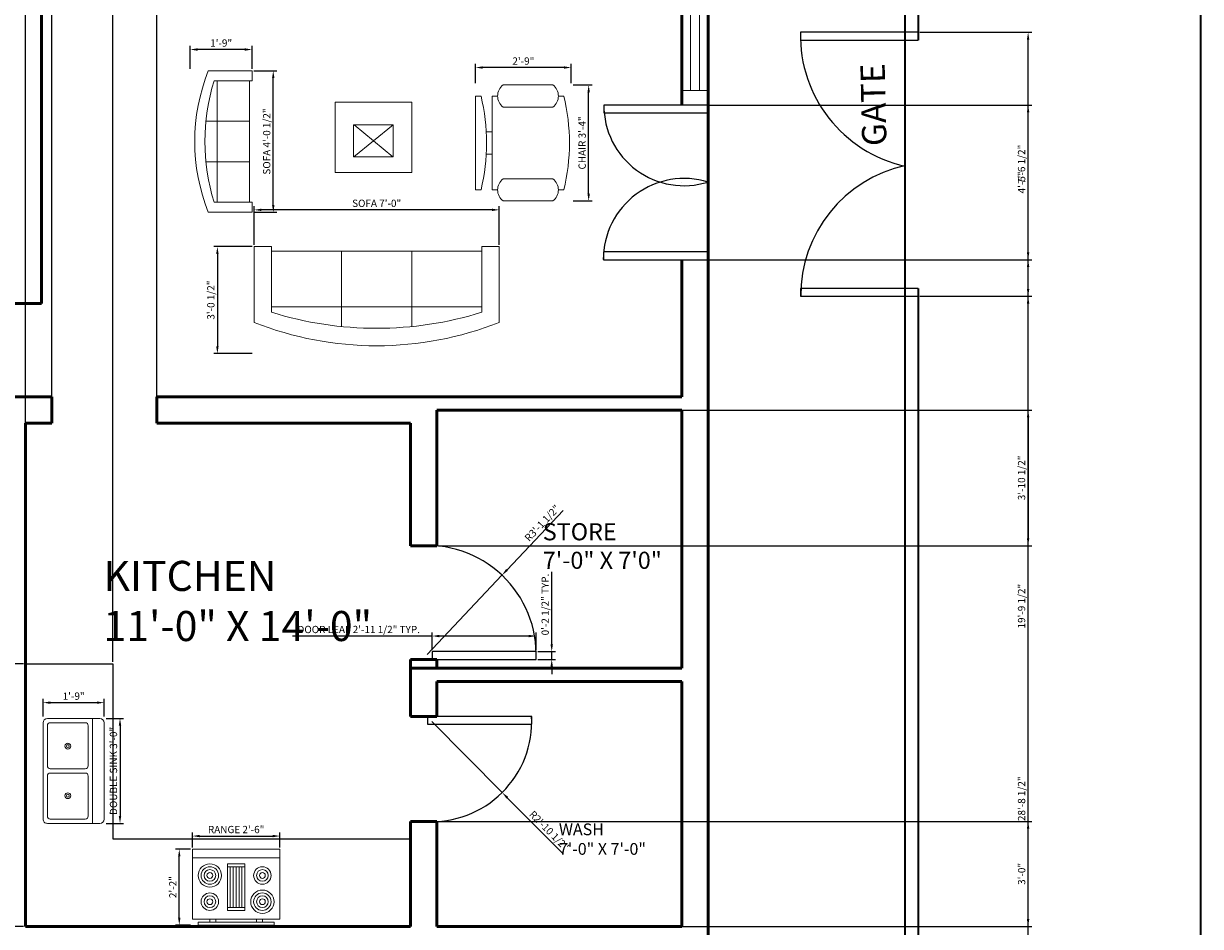
# Model space of a CAD drawing. Units: inches. Extents: x 65 to 818, y -87 to 880.
# Tile 4 of 6: x 414 to 818, y 148 to 457. Entities that reach past the tile are written whole.
import ezdxf

# ---------------------------------------------------------------- set-up
doc = ezdxf.new("R2010")
doc.units = ezdxf.units.IN
for name, color, linetype, lineweight in [('A-ANNO-DIMS', 2, 'Continuous', 18), ('A-ANNO-TEXT', 7, 'Continuous', 25), ('A-ANNO-TTLB', 7, 'Continuous', 35), ('A-AREA-IDEN', 7, 'Continuous', 25), ('A-DOOR', 3, 'Continuous', 25), ('A-EQPM', 9, 'Continuous', 18), ('A-FLOR-CASE', 32, 'Continuous', 25), ('A-FLOR-FIXT', 9, 'Continuous', 18), ('A-FURN', 8, 'Continuous', 18), ('A-GLAZ', 4, 'Continuous', 18), ('A-WALL', 7, 'Continuous', 50), ('C-PROP', 7, 'Continuous', 35), ('L-SITE-GATE', 3, 'Continuous', 25)]:
    doc.layers.add(name, color=color, linetype=linetype, lineweight=lineweight)
doc.styles.get("Standard").update_dxf_attribs({"font": 'arial.ttf'})
doc.dimstyles.new('ISO-25', dxfattribs={"dimtxt": 2.5, "dimasz": 2.5, "dimexe": 1.25, "dimexo": 0.625, "dimtad": 1, "dimtxsty": 'Standard', "dimcen": 2.5, "dimadec": 0, "dimazin": 0, "dimtfac": 1, "dimtmove": 0, "dimatfit": 3, "dimfxl": 1, "dimarcsym": 0})

# ---------------------------------------------------------------- blocks, each defined once
blk = doc.blocks.new('Range-Oven - 30 in top')
for p, q in [((0, -3), (30, -3)), ((12, -6), (18, -6)), ((13, -20), (13, -6)), ((14, -6), (14, -20)), ((15, -20), (15, -6)), ((16, -6), (16, -20)), ((17, -20), (17, -6)), ((18, -20), (12, -20)), ((6, -24), (6, -25)), ((8, -25), (8, -24)), ((22, -25), (22, -24)), ((24, -24), (24, -25))]:
    blk.add_line(p, q)
for points in [[(0, -24), (0, 0), (30, 0), (30, -24)], [(12, -21), (12, -5), (18, -5), (18, -21)], [(2, -26), (2, -25), (28, -25), (28, -26)]]:
    blk.add_lwpolyline(points, close=True)
for centre, radius in [((6, -9), 4), ((6, -9), 3), ((6, -9), 2), ((6, -9), 1), ((24, -9), 3), ((24, -9), 2), ((24, -9), 1), ((6, -18), 3), ((6, -18), 2), ((24, -18), 4), ((24, -18), 3), ((24, -18), 2), ((6, -18), 1), ((24, -18), 1)]:
    blk.add_circle(centre, radius)
blk = doc.blocks.new('Sink-double - 36 in top')
for p, q in [((-18, -4), (18, -4)), ((-0.75, -18.5), (-0.75, -6.5)), ((0.75, -6.5), (0.75, -18.5))]:
    blk.add_line(p, q)
for points in [[(-16.5, 0), (16.5, 0)], [(-18, -19.5), (-18, -1.5)], [(18, -1.5), (18, -19.5)], [(-16.5, -18.5), (-16.5, -6.5)], [(-15.5, -5.5), (-1.75, -5.5)], [(1.75, -5.5), (15.5, -5.5)], [(16.5, -6.5), (16.5, -18.5)], [(-1.75, -19.5), (-15.5, -19.5)], [(15.5, -19.5), (1.75, -19.5)], [(16.5, -21), (-16.5, -21)]]:
    blk.add_lwpolyline(points)
for centre, radius in [((-8.5, -12.5), 1), ((-8.5, -12.5), 0.5), ((8.5, -12.5), 1), ((8.5, -12.5), 0.5)]:
    blk.add_circle(centre, radius)
for centre, radius, start, end in [((-16.5, -1.5), 1.5, 90, 180), ((16.5, -1.5), 1.5, 0, 90), ((-15.5, -6.5), 1, 90, 180), ((-1.75, -6.5), 1, 0, 90), ((1.75, -6.5), 1, 90, 180), ((15.5, -6.5), 1, 0, 90), ((-16.5, -19.5), 1.5, 180, 270), ((-15.5, -18.5), 1, 180, 270), ((-1.75, -18.5), 1, 270, 0), ((1.75, -18.5), 1, 180, 270), ((15.5, -18.5), 1, 270, 0), ((16.5, -19.5), 1.5, 270, 0)]:
    blk.add_arc(centre, radius, start, end)
blk = doc.blocks.new('Sofa - Roundback 7 ft.')
for p, q in [((-12.00002, -32.4421), (-12.00003, -6.5971)), ((11.99997, -32.4421), (11.99998, -6.5971)), ((-36.000027, -34), (-36.000027, -11.4696)), ((35.99998, -34), (35.99998, -11.4696)), ((-35.999844, -13.3819), (35.9998, -13.3819)), ((-36.000027, -32.4421), (35.99998, -32.4421))]:
    blk.add_line(p, q)
for points in [[(-36.000027, -34), (-42.000027, -34), (-42.000027, -8)], [(41.99998, -8), (41.99998, -34), (35.99998, -34)]]:
    blk.add_lwpolyline(points)
for centre, radius, start, end in [((0, -114.25), 114.25, 68.43141, 111.5686), ((-0.00001, -127.1968), 121.1968, 72.72033, 107.2797)]:
    blk.add_arc(centre, radius, start, end)
blk = doc.blocks.new('Chair - Desk')
for p, q in [((-8.5, 0), (-8.5, -1)), ((-8.5, 0), (8.5, 0)), ((8.5, 0), (8.5, -1)), ((-2, -3), (-2, -1.9355)), ((2, -1.9576), (2, -3)), ((-8.5, -3), (-8.5, -4)), ((-8.5, -3), (8.5, -3)), ((8.5, -3), (8.5, -4)), ((-10.5, -5), (-10.5, -14)), ((-6.5, -14), (-6.5, -5)), ((6.5, -5), (6.5, -14)), ((10.5, -14), (10.5, -5)), ((-8.5, -15), (-8.5, -16)), ((8.5, -15), (8.5, -16))]:
    blk.add_line(p, q)
for centre, radius, start, end in [((0, 34.625), 36.625, 256.5803, 283.4197), ((-8.5, -6.5), 2.5, 36.8699, 143.1301), ((8.5, -6.5), 2.5, 36.8699, 143.1301), ((-8.5, -12.5), 2.5, 216.8699, 323.1301), ((8.5, -12.5), 2.5, 216.8699, 323.1301), ((0, 19.625), 36.625, 256.5803, 283.4197)]:
    blk.add_arc(centre, radius, start, end)
blk = doc.blocks.new('WIN-52X9-PLAN')
for p, q in [((9, 51.82), (0, 51.82)), ((0, 51.82), (0, 0)), ((3, 0), (3, 51.82)), ((6, 51.82), (6, 0)), ((9, 0), (9, 51.82)), ((0, 0), (9, 0))]:
    blk.add_line(p, q)
blk = doc.blocks.new('DOOR-LEAF-36-NOM')
blk.add_lwpolyline([(0, 0), (2.67, 0), (2.67, 35.67), (0, 35.67)], close=True)
blk = doc.blocks.new('*D18')
at = {"layer": 'A-ANNO-DIMS', "color": 0, "lineweight": -2, "transparency": 16777216}
for p, q in [((554.18, 247.07), (506.39, 247.07)), ((554.18, 242.34), (554.18, 248.32)), ((587.35, 247.07), (556.68, 247.07)), ((589.85, 242.34), (589.85, 248.32))]:
    blk.add_line(p, q, dxfattribs=at)
at = {"layer": 'A-ANNO-DIMS', "color": 0, "transparency": 16777216}
for points in [[(556.68, 247.48), (556.68, 246.65), (554.18, 247.07)], [(587.35, 247.48), (587.35, 246.65), (589.85, 247.07)]]:
    blk.add_solid(points, dxfattribs=at)
at = {"layer": 'Defpoints', "color": 0, "transparency": 16777216}
for p in [(554.18, 247.07), (554.18, 241.72), (589.85, 241.72)]:
    blk.add_point(p, dxfattribs=at)
at = {"layer": 'A-ANNO-DIMS', "color": 0, "transparency": 16777216, "insert": (529.04, 248.99), "char_height": 2.5, "attachment_point": 5}
blk.add_mtext('DOOR LEAF 2\'-11 1/2" TYP.', dxfattribs=at)
blk = doc.blocks.new('*D19')
at = {"layer": 'A-ANNO-DIMS', "color": 0, "lineweight": -2, "transparency": 16777216}
for p, q in [((595.2, 244.22), (595.2, 269.03)), ((590.47, 241.72), (596.45, 241.72)), ((590.47, 239.05), (596.45, 239.05)), ((595.2, 239.05), (595.2, 241.72)), ((595.2, 236.55), (595.2, 234.05))]:
    blk.add_line(p, q, dxfattribs=at)
at = {"layer": 'A-ANNO-DIMS', "color": 0, "transparency": 16777216}
for points in [[(594.78, 244.22), (595.61, 244.22), (595.2, 241.72)], [(594.78, 236.55), (595.61, 236.55), (595.2, 239.05)]]:
    blk.add_solid(points, dxfattribs=at)
at = {"layer": 'Defpoints', "color": 0, "transparency": 16777216}
for p in [(589.85, 241.72), (589.85, 239.05), (595.2, 241.72)]:
    blk.add_point(p, dxfattribs=at)
at = {"layer": 'A-ANNO-DIMS', "color": 0, "transparency": 16777216, "insert": (593.28, 257.87), "char_height": 2.5, "attachment_point": 5, "rotation": 90}
blk.add_mtext('0\'-2 1/2" TYP.', dxfattribs=at)
blk = doc.blocks.new('*D36')
at = {"layer": 'A-ANNO-DIMS', "color": 0, "lineweight": -2, "transparency": 16777216}
for p, q in [((493.19, 381.19), (493.19, 394.42)), ((574.69, 393.17), (495.69, 393.17)), ((577.19, 381.19), (577.19, 394.42))]:
    blk.add_line(p, q, dxfattribs=at)
at = {"layer": 'A-ANNO-DIMS', "color": 0, "transparency": 16777216}
for points in [[(495.69, 393.58), (495.69, 392.75), (493.19, 393.17)], [(574.69, 393.58), (574.69, 392.75), (577.19, 393.17)]]:
    blk.add_solid(points, dxfattribs=at)
at = {"layer": 'Defpoints', "color": 0, "transparency": 16777216}
for p in [(493.19, 393.17), (493.19, 380.57), (577.19, 380.57)]:
    blk.add_point(p, dxfattribs=at)
at = {"layer": 'A-ANNO-DIMS', "color": 0, "transparency": 16777216, "insert": (535.19, 395.08), "char_height": 2.5, "attachment_point": 5}
blk.add_mtext('SOFA 7\'-0"', dxfattribs=at)
blk = doc.blocks.new('*D37')
at = {"layer": 'A-ANNO-DIMS', "color": 0, "lineweight": -2, "transparency": 16777216}
for p, q in [((492.56, 380.57), (479.34, 380.57)), ((480.59, 378.07), (480.59, 346.4)), ((492.56, 343.9), (479.34, 343.9))]:
    blk.add_line(p, q, dxfattribs=at)
at = {"layer": 'A-ANNO-DIMS', "color": 0, "transparency": 16777216}
for points in [[(480.17, 378.07), (481.01, 378.07), (480.59, 380.57)], [(480.17, 346.4), (481.01, 346.4), (480.59, 343.9)]]:
    blk.add_solid(points, dxfattribs=at)
at = {"layer": 'Defpoints', "color": 0, "transparency": 16777216}
for p in [(493.19, 380.57), (480.59, 343.9), (493.19, 343.9)]:
    blk.add_point(p, dxfattribs=at)
at = {"layer": 'A-ANNO-DIMS', "color": 0, "transparency": 16777216, "insert": (478.67, 362.23), "char_height": 2.5, "attachment_point": 5, "rotation": 90}
blk.add_mtext('3\'-0 1/2"', dxfattribs=at)
blk = doc.blocks.new('*D38')
at = {"layer": 'A-ANNO-DIMS', "color": 0, "lineweight": -2, "transparency": 16777216}
for p, q in [((493.09, 440.84), (500.99, 440.84)), ((499.74, 394.83), (499.74, 438.34)), ((493.09, 392.33), (500.99, 392.33))]:
    blk.add_line(p, q, dxfattribs=at)
at = {"layer": 'A-ANNO-DIMS', "color": 0, "transparency": 16777216}
for points in [[(499.33, 438.34), (500.16, 438.34), (499.74, 440.84)], [(499.33, 394.83), (500.16, 394.83), (499.74, 392.33)]]:
    blk.add_solid(points, dxfattribs=at)
at = {"layer": 'Defpoints', "color": 0, "transparency": 16777216}
for p in [(492.47, 440.84), (499.74, 440.84), (492.47, 392.33)]:
    blk.add_point(p, dxfattribs=at)
at = {"layer": 'A-ANNO-DIMS', "color": 0, "transparency": 16777216, "insert": (497.82, 416.59), "char_height": 2.5, "attachment_point": 5, "rotation": 90}
blk.add_mtext('SOFA 4\'-0 1/2"', dxfattribs=at)
blk = doc.blocks.new('*D39')
at = {"layer": 'A-ANNO-DIMS', "color": 0, "lineweight": -2, "transparency": 16777216}
for p, q in [((471.29, 441.47), (471.29, 449.37)), ((489.97, 448.12), (473.79, 448.12)), ((492.47, 441.47), (492.47, 449.37))]:
    blk.add_line(p, q, dxfattribs=at)
at = {"layer": 'A-ANNO-DIMS', "color": 0, "transparency": 16777216}
for points in [[(473.79, 448.54), (473.79, 447.7), (471.29, 448.12)], [(489.97, 448.54), (489.97, 447.7), (492.47, 448.12)]]:
    blk.add_solid(points, dxfattribs=at)
at = {"layer": 'Defpoints', "color": 0, "transparency": 16777216}
for p in [(471.29, 448.12), (471.29, 440.84), (492.47, 440.84)]:
    blk.add_point(p, dxfattribs=at)
at = {"layer": 'A-ANNO-DIMS', "color": 0, "transparency": 16777216, "insert": (481.88, 450.02), "char_height": 2.5, "attachment_point": 5}
blk.add_mtext('1\'-9"', dxfattribs=at)
blk = doc.blocks.new('*D42')
at = {"layer": 'A-ANNO-DIMS', "color": 0, "lineweight": -2, "transparency": 16777216}
for p, q in [((472.02, 174.63), (472.02, 179.75)), ((474.52, 178.5), (499.52, 178.5)), ((502.02, 174.63), (502.02, 179.75))]:
    blk.add_line(p, q, dxfattribs=at)
at = {"layer": 'A-ANNO-DIMS', "color": 0, "transparency": 16777216}
for points in [[(474.52, 178.92), (474.52, 178.09), (472.02, 178.5)], [(499.52, 178.92), (499.52, 178.09), (502.02, 178.5)]]:
    blk.add_solid(points, dxfattribs=at)
at = {"layer": 'Defpoints', "color": 0, "transparency": 16777216}
for p in [(502.02, 178.5), (472.02, 174), (502.02, 174)]:
    blk.add_point(p, dxfattribs=at)
at = {"layer": 'A-ANNO-DIMS', "color": 0, "transparency": 16777216, "insert": (487.02, 180.42), "char_height": 2.5, "attachment_point": 5}
blk.add_mtext('RANGE 2\'-6"', dxfattribs=at)
blk = doc.blocks.new('*D43')
at = {"layer": 'A-ANNO-DIMS', "color": 0, "lineweight": -2, "transparency": 16777216}
for p, q in [((471.4, 174), (466.27, 174)), ((467.52, 150.5), (467.52, 171.5)), ((471.4, 148), (466.27, 148))]:
    blk.add_line(p, q, dxfattribs=at)
at = {"layer": 'A-ANNO-DIMS', "color": 0, "transparency": 16777216}
for points in [[(467.11, 171.5), (467.94, 171.5), (467.52, 174)], [(467.11, 150.5), (467.94, 150.5), (467.52, 148)]]:
    blk.add_solid(points, dxfattribs=at)
at = {"layer": 'Defpoints', "color": 0, "transparency": 16777216}
for p in [(467.52, 174), (472.02, 174), (472.02, 148)]:
    blk.add_point(p, dxfattribs=at)
at = {"layer": 'A-ANNO-DIMS', "color": 0, "transparency": 16777216, "insert": (465.64, 161), "char_height": 2.5, "attachment_point": 5, "rotation": 90}
blk.add_mtext('2\'-2"', dxfattribs=at)
blk = doc.blocks.new('*D44')
at = {"layer": 'A-ANNO-DIMS', "color": 0, "lineweight": -2, "transparency": 16777216}
for p, q in [((442.43, 218.84), (448.46, 218.84)), ((447.21, 216.34), (447.21, 185.34)), ((442.43, 182.84), (448.46, 182.84))]:
    blk.add_line(p, q, dxfattribs=at)
at = {"layer": 'A-ANNO-DIMS', "color": 0, "transparency": 16777216}
for points in [[(446.79, 216.34), (447.62, 216.34), (447.21, 218.84)], [(446.79, 185.34), (447.62, 185.34), (447.21, 182.84)]]:
    blk.add_solid(points, dxfattribs=at)
at = {"layer": 'Defpoints', "color": 0, "transparency": 16777216}
for p in [(441.81, 218.84), (441.81, 182.84), (447.21, 182.84)]:
    blk.add_point(p, dxfattribs=at)
at = {"layer": 'A-ANNO-DIMS', "color": 0, "transparency": 16777216, "insert": (445.29, 200.84), "char_height": 2.5, "attachment_point": 5, "rotation": 90}
blk.add_mtext('DOUBLE SINK 3\'-0"', dxfattribs=at)
blk = doc.blocks.new('*D45')
at = {"layer": 'A-ANNO-DIMS', "color": 0, "lineweight": -2, "transparency": 16777216}
for p, q in [((420.81, 219.46), (420.81, 225.49)), ((423.31, 224.24), (439.31, 224.24)), ((441.81, 219.46), (441.81, 225.49))]:
    blk.add_line(p, q, dxfattribs=at)
at = {"layer": 'A-ANNO-DIMS', "color": 0, "transparency": 16777216}
for points in [[(423.31, 224.65), (423.31, 223.82), (420.81, 224.24)], [(439.31, 224.65), (439.31, 223.82), (441.81, 224.24)]]:
    blk.add_solid(points, dxfattribs=at)
at = {"layer": 'Defpoints', "color": 0, "transparency": 16777216}
for p in [(441.81, 224.24), (420.81, 218.84), (441.81, 218.84)]:
    blk.add_point(p, dxfattribs=at)
at = {"layer": 'A-ANNO-DIMS', "color": 0, "transparency": 16777216, "insert": (431.31, 226.14), "char_height": 2.5, "attachment_point": 5}
blk.add_mtext('1\'-9"', dxfattribs=at)
blk = doc.blocks.new('*D46')
at = {"layer": 'A-ANNO-DIMS', "color": 0, "lineweight": -2, "transparency": 16777216}
for p, q in [((602.52, 435.98), (609.11, 435.98)), ((607.86, 398.7), (607.86, 433.48)), ((602.52, 396.2), (609.11, 396.2))]:
    blk.add_line(p, q, dxfattribs=at)
at = {"layer": 'A-ANNO-DIMS', "color": 0, "transparency": 16777216}
for points in [[(607.45, 433.48), (608.28, 433.48), (607.86, 435.98)], [(607.45, 398.7), (608.28, 398.7), (607.86, 396.2)]]:
    blk.add_solid(points, dxfattribs=at)
at = {"layer": 'Defpoints', "color": 0, "transparency": 16777216}
for p in [(601.9, 435.98), (607.86, 435.98), (601.9, 396.2)]:
    blk.add_point(p, dxfattribs=at)
at = {"layer": 'A-ANNO-DIMS', "color": 0, "transparency": 16777216, "insert": (605.95, 416.09), "char_height": 2.5, "attachment_point": 5, "rotation": 90}
blk.add_mtext('CHAIR 3\'-4"', dxfattribs=at)
blk = doc.blocks.new('*D47')
at = {"layer": 'A-ANNO-DIMS', "color": 0, "lineweight": -2, "transparency": 16777216}
for p, q in [((569.07, 436.6), (569.07, 443.2)), ((599.4, 441.95), (571.57, 441.95)), ((601.9, 436.6), (601.9, 443.2))]:
    blk.add_line(p, q, dxfattribs=at)
at = {"layer": 'A-ANNO-DIMS', "color": 0, "transparency": 16777216}
for points in [[(571.57, 442.36), (571.57, 441.53), (569.07, 441.95)], [(599.4, 442.36), (599.4, 441.53), (601.9, 441.95)]]:
    blk.add_solid(points, dxfattribs=at)
at = {"layer": 'Defpoints', "color": 0, "transparency": 16777216}
for p in [(569.07, 441.95), (569.07, 435.98), (601.9, 435.98)]:
    blk.add_point(p, dxfattribs=at)
at = {"layer": 'A-ANNO-DIMS', "color": 0, "transparency": 16777216, "insert": (585.48, 443.85), "char_height": 2.5, "attachment_point": 5}
blk.add_mtext('2\'-9"', dxfattribs=at)
blk = doc.blocks.new('*D55')
at = {"layer": 'A-ANNO-DIMS', "color": 0, "lineweight": -2, "transparency": 16777216}
for p, q in [((721.42, 454.02), (759.75, 454.02)), ((758.5, 366.05), (758.5, 451.52)), ((721.42, 363.55), (759.75, 363.55))]:
    blk.add_line(p, q, dxfattribs=at)
at = {"layer": 'A-ANNO-DIMS', "color": 0, "transparency": 16777216}
for points in [[(758.08, 451.52), (758.92, 451.52), (758.5, 454.02)], [(758.08, 366.05), (758.92, 366.05), (758.5, 363.55)]]:
    blk.add_solid(points, dxfattribs=at)
at = {"layer": 'Defpoints', "color": 0, "transparency": 16777216}
for p in [(720.8, 454.02), (758.5, 454.02), (720.8, 363.55)]:
    blk.add_point(p, dxfattribs=at)
at = {"layer": 'A-ANNO-DIMS', "color": 0, "transparency": 16777216, "insert": (756.58, 408.79), "char_height": 2.5, "attachment_point": 5, "rotation": 90}
blk.add_mtext('7\'-6 1/2"', dxfattribs=at)
blk = doc.blocks.new('*D56')
at = {"layer": 'A-ANNO-DIMS', "color": 0, "lineweight": -2, "transparency": 16777216}
for p, q in [((649.42, 429.07), (759.75, 429.07)), ((758.5, 378.58), (758.5, 426.57)), ((649.42, 376.08), (759.75, 376.08))]:
    blk.add_line(p, q, dxfattribs=at)
at = {"layer": 'A-ANNO-DIMS', "color": 0, "transparency": 16777216}
for points in [[(758.08, 426.57), (758.92, 426.57), (758.5, 429.07)], [(758.08, 378.58), (758.92, 378.58), (758.5, 376.08)]]:
    blk.add_solid(points, dxfattribs=at)
at = {"layer": 'Defpoints', "color": 0, "transparency": 16777216}
for p in [(648.8, 429.07), (758.5, 429.07), (648.8, 376.08)]:
    blk.add_point(p, dxfattribs=at)
at = {"layer": 'A-ANNO-DIMS', "color": 0, "transparency": 16777216, "insert": (756.6, 402.57), "char_height": 2.5, "attachment_point": 5, "rotation": 90}
blk.add_mtext('4\'-5"', dxfattribs=at)
blk = doc.blocks.new('*D58')
at = {"layer": 'A-ANNO-DIMS', "color": 0, "lineweight": -2, "transparency": 16777216}
for p, q in [((414.8, 238.17), (414.8, 777.99)), ((417.3, 776.74), (442.3, 776.74)), ((444.8, 238.17), (444.8, 777.99))]:
    blk.add_line(p, q, dxfattribs=at)
at = {"layer": 'A-ANNO-DIMS', "color": 0, "transparency": 16777216}
for points in [[(417.3, 777.16), (417.3, 776.32), (414.8, 776.74)], [(442.3, 777.16), (442.3, 776.32), (444.8, 776.74)]]:
    blk.add_solid(points, dxfattribs=at)
at = {"layer": 'Defpoints', "color": 0, "transparency": 16777216}
for p in [(444.8, 776.74), (414.8, 237.54), (444.8, 237.54)]:
    blk.add_point(p, dxfattribs=at)
at = {"layer": 'A-ANNO-DIMS', "color": 0, "transparency": 16777216, "insert": (429.8, 778.64), "char_height": 2.5, "attachment_point": 5}
blk.add_mtext('2\'-6"', dxfattribs=at)
blk = doc.blocks.new('*D60')
at = {"layer": 'A-ANNO-DIMS', "color": 0, "lineweight": -2, "transparency": 16777216}
for p, q in [((649.42, 376.08), (759.75, 376.08)), ((758.5, 141.04), (758.5, 373.58)), ((649.42, 138.54), (759.75, 138.54))]:
    blk.add_line(p, q, dxfattribs=at)
at = {"layer": 'A-ANNO-DIMS', "color": 0, "transparency": 16777216}
for points in [[(758.08, 373.58), (758.92, 373.58), (758.5, 376.08)], [(758.08, 141.04), (758.92, 141.04), (758.5, 138.54)]]:
    blk.add_solid(points, dxfattribs=at)
at = {"layer": 'Defpoints', "color": 0, "transparency": 16777216}
for p in [(648.8, 376.08), (758.5, 376.08), (648.8, 138.54)]:
    blk.add_point(p, dxfattribs=at)
at = {"layer": 'A-ANNO-DIMS', "color": 0, "transparency": 16777216, "insert": (756.58, 257.31), "char_height": 2.5, "attachment_point": 5, "rotation": 90}
blk.add_mtext('19\'-9 1/2"', dxfattribs=at)
blk = doc.blocks.new('*D65')
at = {"layer": 'A-ANNO-DIMS', "color": 0, "lineweight": -2, "transparency": 16777216}
for p, q in [((721.42, 363.55), (759.75, 363.55)), ((758.5, 21.54), (758.5, 361.05)), ((721.42, 19.04), (759.75, 19.04))]:
    blk.add_line(p, q, dxfattribs=at)
at = {"layer": 'A-ANNO-DIMS', "color": 0, "transparency": 16777216}
for points in [[(758.08, 361.05), (758.92, 361.05), (758.5, 363.55)], [(758.08, 21.54), (758.92, 21.54), (758.5, 19.04)]]:
    blk.add_solid(points, dxfattribs=at)
at = {"layer": 'Defpoints', "color": 0, "transparency": 16777216}
for p in [(720.8, 363.55), (758.5, 363.55), (720.8, 19.04)]:
    blk.add_point(p, dxfattribs=at)
at = {"layer": 'A-ANNO-DIMS', "color": 0, "transparency": 16777216, "insert": (756.58, 191.3), "char_height": 2.5, "attachment_point": 5, "rotation": 90}
blk.add_mtext('28\'-8 1/2"', dxfattribs=at)
blk = doc.blocks.new('*D66')
at = {"layer": 'A-ANNO-DIMS', "color": 0, "lineweight": -2, "transparency": 16777216}
for p, q in [((423.8, 320.67), (423.8, 777.99)), ((426.3, 776.74), (457.3, 776.74)), ((459.8, 320.67), (459.8, 777.99))]:
    blk.add_line(p, q, dxfattribs=at)
at = {"layer": 'A-ANNO-DIMS', "color": 0, "transparency": 16777216}
for points in [[(426.3, 777.16), (426.3, 776.32), (423.8, 776.74)], [(457.3, 777.16), (457.3, 776.32), (459.8, 776.74)]]:
    blk.add_solid(points, dxfattribs=at)
at = {"layer": 'Defpoints', "color": 0, "transparency": 16777216}
for p in [(459.8, 776.74), (423.8, 320.04), (459.8, 320.04)]:
    blk.add_point(p, dxfattribs=at)
at = {"layer": 'A-ANNO-DIMS', "color": 0, "transparency": 16777216, "insert": (441.8, 778.64), "char_height": 2.5, "attachment_point": 5}
blk.add_mtext('3\'-0"', dxfattribs=at)
blk = doc.blocks.new('*D69')
at = {"layer": 'A-ANNO-DIMS', "color": 0, "lineweight": -2, "transparency": 16777216}
for p, q in [((556.42, 183.54), (759.75, 183.54)), ((758.5, 150.04), (758.5, 181.04)), ((556.42, 147.54), (759.75, 147.54))]:
    blk.add_line(p, q, dxfattribs=at)
at = {"layer": 'A-ANNO-DIMS', "color": 0, "transparency": 16777216}
for points in [[(758.08, 181.04), (758.92, 181.04), (758.5, 183.54)], [(758.08, 150.04), (758.92, 150.04), (758.5, 147.54)]]:
    blk.add_solid(points, dxfattribs=at)
at = {"layer": 'Defpoints', "color": 0, "transparency": 16777216}
for p in [(555.8, 183.54), (758.5, 183.54), (555.8, 147.54)]:
    blk.add_point(p, dxfattribs=at)
at = {"layer": 'A-ANNO-DIMS', "color": 0, "transparency": 16777216, "insert": (756.6, 165.54), "char_height": 2.5, "attachment_point": 5, "rotation": 90}
blk.add_mtext('3\'-0"', dxfattribs=at)
blk = doc.blocks.new('*D70')
at = {"layer": 'A-ANNO-DIMS', "color": 0, "lineweight": -2, "transparency": 16777216}
for p, q in [((556.42, 324.54), (759.75, 324.54)), ((758.5, 322.04), (758.5, 280.54)), ((556.42, 278.04), (759.75, 278.04))]:
    blk.add_line(p, q, dxfattribs=at)
at = {"layer": 'A-ANNO-DIMS', "color": 0, "transparency": 16777216}
for points in [[(758.08, 322.04), (758.92, 322.04), (758.5, 324.54)], [(758.08, 280.54), (758.92, 280.54), (758.5, 278.04)]]:
    blk.add_solid(points, dxfattribs=at)
at = {"layer": 'Defpoints', "color": 0, "transparency": 16777216}
for p in [(555.8, 324.54), (555.8, 278.04), (758.5, 278.04)]:
    blk.add_point(p, dxfattribs=at)
at = {"layer": 'A-ANNO-DIMS', "color": 0, "transparency": 16777216, "insert": (756.58, 301.29), "char_height": 2.5, "attachment_point": 5, "rotation": 90}
blk.add_mtext('3\'-10 1/2"', dxfattribs=at)
blk = doc.blocks.new('*D74')
at = {"layer": 'A-ANNO-DIMS', "color": 0, "lineweight": -2, "transparency": 16777216}
for p, q in [((414.17, 237.54), (201.85, 237.54)), ((203.1, 150.04), (203.1, 235.04)), ((414.17, 147.54), (201.85, 147.54))]:
    blk.add_line(p, q, dxfattribs=at)
at = {"layer": 'A-ANNO-DIMS', "color": 0, "transparency": 16777216}
for points in [[(202.68, 235.04), (203.52, 235.04), (203.1, 237.54)], [(202.68, 150.04), (203.52, 150.04), (203.1, 147.54)]]:
    blk.add_solid(points, dxfattribs=at)
at = {"layer": 'Defpoints', "color": 0, "transparency": 16777216}
for p in [(203.1, 237.54), (414.8, 237.54), (414.8, 147.54)]:
    blk.add_point(p, dxfattribs=at)
at = {"layer": 'A-ANNO-DIMS', "color": 0, "transparency": 16777216, "insert": (201.2, 192.54), "char_height": 2.5, "attachment_point": 5, "rotation": 90}
blk.add_mtext('7\'-6"', dxfattribs=at)
blk = doc.blocks.new('*D78')
at = {"layer": 'A-ANNO-DIMS', "color": 0, "lineweight": -2, "transparency": 16777216}
for p, q in [((554.06, 217.78), (578.22, 193.43)), ((599.07, 172.4), (579.98, 191.65))]:
    blk.add_line(p, q, dxfattribs=at)
at = {"layer": 'A-ANNO-DIMS', "color": 0, "transparency": 16777216}
blk.add_solid([(580.27, 191.94), (579.68, 191.36), (578.22, 193.43)], dxfattribs=at)
at = {"layer": 'Defpoints', "color": 0, "transparency": 16777216}
for p in [(554.06, 217.78), (578.22, 193.43)]:
    blk.add_point(p, dxfattribs=at)
at = {"layer": 'A-ANNO-DIMS', "color": 0, "transparency": 16777216, "insert": (594.07, 180.16), "char_height": 2.5, "attachment_point": 5, "rotation": 314.7642}
blk.add_mtext('R2\'-10 1/2"', dxfattribs=at)
blk = doc.blocks.new('*D82')
at = {"layer": 'A-ANNO-DIMS', "color": 0, "lineweight": -2, "transparency": 16777216}
for p, q in [((599.09, 290.1), (579.87, 269.74)), ((552.47, 240.73), (578.15, 267.92))]:
    blk.add_line(p, q, dxfattribs=at)
at = {"layer": 'A-ANNO-DIMS', "color": 0, "transparency": 16777216}
blk.add_solid([(579.56, 270.03), (580.17, 269.45), (578.15, 267.92)], dxfattribs=at)
at = {"layer": 'Defpoints', "color": 0, "transparency": 16777216}
for p in [(578.15, 267.92), (552.47, 240.73)]:
    blk.add_point(p, dxfattribs=at)
at = {"layer": 'A-ANNO-DIMS', "color": 0, "transparency": 16777216, "insert": (592.16, 285.56), "char_height": 2.5, "attachment_point": 5, "rotation": 46.6417}
blk.add_mtext('R3\'-1 1/2"', dxfattribs=at)

msp = doc.modelspace()

# ---------------------------------------------------------------- linework, layer by layer
at = {"layer": 'A-ANNO-TTLB'}
msp.add_lwpolyline([(64.55, 880.46), (817.59, 880.46), (817.59, -87.37), (64.55, -87.37)], close=True, dxfattribs=at)
at = {"layer": 'A-DOOR'}
for points in [[(648.8, 429.07), (613.08, 429.07), (613.08, 426.4), (648.8, 426.41)], [(648.8, 378.74), (612.9, 378.74), (612.9, 376.08), (648.8, 376.08)]]:
    msp.add_lwpolyline(points, dxfattribs=at)
for centre, radius, start, end in [((640.55, 428.93), 27.49, 179.6774, 287.4638), ((640.61, 376.17), 27.75, 72.8481, 180.1098), ((552.47, 240.73), 37.41, 357.4133, 95.8708), ((554.06, 217.78), 34.3, 266.6167, 2.9116)]:
    msp.add_arc(centre, radius, start, end, dxfattribs=at)
at = {"layer": 'A-FLOR-CASE'}
for p, q in [((414.8, 237.54), (444.8, 237.54)), ((444.8, 237.54), (444.8, 177.54)), ((444.8, 177.54), (546.8, 177.54))]:
    msp.add_line(p, q, dxfattribs=at)
at = {"layer": 'A-FURN'}
for p, q in [((527.33, 411.31), (540.79, 422.27)), ((540.72, 411.35), (527.49, 422.28))]:
    msp.add_line(p, q, dxfattribs=at)
for points in [[(520.92, 430.08), (547.26, 430.08), (547.26, 405.92), (520.92, 405.92)], [(527.3, 422.28), (540.79, 422.28), (540.79, 411.35), (527.3, 411.35)]]:
    msp.add_lwpolyline(points, close=True, dxfattribs=at)
at = {"layer": 'A-WALL'}
for p, q in [((648.8, 703.04), (648.8, 138.54)), ((639.8, 517.04), (639.8, 429.07)), ((420.3, 361.04), (420.3, 460.04)), ((639.8, 402.69), (639.8, 402.69)), ((639.8, 376.08), (639.8, 329.04)), ((374.3, 361.04), (420.3, 361.04)), ((405.8, 329.04), (423.8, 329.04)), ((423.8, 329.04), (423.8, 320.04)), ((459.8, 329.04), (459.8, 320.04)), ((459.8, 329.04), (639.8, 329.04)), ((555.8, 324.54), (639.8, 324.54)), ((555.8, 324.54), (555.8, 278.04)), ((639.8, 324.54), (639.8, 236.04)), ((414.8, 320.04), (423.8, 320.04)), ((414.8, 320.04), (414.8, 147.54)), ((459.8, 320.04), (546.8, 320.04)), ((546.8, 320.04), (546.8, 278.04)), ((546.8, 278.04), (555.8, 278.04)), ((546.8, 239.04), (555.8, 239.04)), ((546.8, 239.04), (546.8, 219.54)), ((555.8, 239.04), (555.8, 236.04)), ((546.8, 236.04), (639.8, 236.04)), ((555.8, 231.54), (639.8, 231.54)), ((555.8, 231.54), (555.8, 219.54)), ((639.8, 231.54), (639.8, 147.54)), ((546.8, 219.54), (555.8, 219.54)), ((546.8, 183.54), (555.8, 183.54)), ((546.8, 183.54), (546.8, 147.54)), ((555.8, 183.54), (555.8, 147.54)), ((414.8, 147.54), (546.8, 147.54)), ((555.8, 147.54), (639.8, 147.54))]:
    msp.add_line(p, q, dxfattribs=at)
at = {"layer": 'C-PROP'}
for p, q in [((720.8, 739.04), (720.8, 451.35)), ((716.3, 734.54), (716.3, 23.54)), ((720.8, 366.22), (720.8, 19.04))]:
    msp.add_line(p, q, dxfattribs=at)
at = {"layer": 'L-SITE-GATE'}
for points in [[(720.8, 454.02), (680.47, 454.02), (680.47, 451.35), (720.8, 451.35)], [(720.8, 366.22), (680.47, 366.22), (680.47, 363.55), (720.8, 363.55)]]:
    msp.add_lwpolyline(points, dxfattribs=at)
for centre, radius, start, end in [((726.32, 452.93), 45.87, 178.7141, 257.4649), ((726.08, 363.86), 45.53, 102.1735, 180.4965)]:
    msp.add_arc(centre, radius, start, end, dxfattribs=at)

# ---------------------------------------------------------------- block references
at = {"layer": 'A-DOOR', "rotation": 90.00000000000007}
for p in [(589.85, 239.05), (588.34, 216.87)]:
    msp.add_blockref('DOOR-LEAF-36-NOM', p, dxfattribs=at)
at = {"layer": 'A-EQPM'}
msp.add_blockref('Range-Oven - 30 in top', (472.02, 174), dxfattribs=at)
at = {"layer": 'A-FLOR-FIXT', "rotation": 270}
msp.add_blockref('Sink-double - 36 in top', (441.81, 200.84), dxfattribs=at)
at = {"layer": 'A-FURN'}
for name, p, xscale, yscale, zscale, rotation in [('Sofa - Roundback 7 ft.', (472.83, 416.59), 0.5775366576221616, 0.5775366576221616, 0.5775366576221616, 89.99999999999999), ('Chair - Desk', (569.07, 416.09), 1.894169593508299, 1.894169593508299, 1.894169593508299, 90)]:
    msp.add_blockref(name, p, dxfattribs=dict(at, xscale=xscale, yscale=yscale, zscale=zscale, rotation=rotation))
at = {"layer": 'A-FURN', "rotation": 180}
msp.add_blockref('Sofa - Roundback 7 ft.', (535.19, 346.57), dxfattribs=at)
at = {"layer": 'A-GLAZ'}
msp.add_blockref('WIN-52X9-PLAN', (639.8, 434.13), dxfattribs=at)

# ---------------------------------------------------------------- texts
at = {"layer": 'A-ANNO-TEXT', "insert": (701.64, 414.94), "char_height": 8.353, "attachment_point": 1, "rotation": 91.3254}
msp.add_mtext_dynamic_manual_height_columns('GATE', width=13.7685, gutter_width=41.77, heights=[0], dxfattribs=at)
at = {"layer": 'A-AREA-IDEN', "attachment_point": 1}
for s, width, gutter_width, insert, char_height in [('STORE\\P7\'-0" X 7\'0"', 90.223, 29.37, (592.14, 285.76), 5.8749), ('KITCHEN\\P11\'-0" X 14\'-0"', 100.5512, 51.51, (441.56, 272.83), 10.3025), ('WASH\\P7\'-0" X 7\'-0"', 31.7279, 20.11, (597.66, 182.81), 4.0221)]:
    msp.add_mtext_dynamic_manual_height_columns(s, width=width, gutter_width=gutter_width, heights=[0], dxfattribs=dict(at, insert=insert, char_height=char_height))

# ---------------------------------------------------------------- dimensions: what is measured, and where the dimension line sits
at = {"layer": 'A-ANNO-DIMS'}
for base, p1, p2, picture, middle in [((444.8, 776.74), (414.8, 237.54), (444.8, 237.54), '*D58', (429.8, 778.64)), ((459.8, 776.74), (423.8, 320.04), (459.8, 320.04), '*D66', (441.8, 778.64)), ((441.81, 224.24), (420.81, 218.84), (441.81, 218.84), '*D45', (431.31, 226.14))]:
    dim = msp.add_linear_dim(base=base, p1=p1, p2=p2, dimstyle='ISO-25', override={"dimdec": 1, "dimlfac": 1, "dimrnd": 0, "dimzin": 1, "dimdsep": 46, "dimlunit": 4, "dimfrac": 2}, dxfattribs=at)
    dim.commit()
    dim.dimension.update_dxf_attribs({"geometry": picture, "text_midpoint": middle})
for base, p1, p2, angle, picture, middle in [((758.5, 454.02), (720.8, 363.55), (720.8, 454.02), 90, '*D55', (756.58, 408.79)), ((471.29, 448.12), (492.47, 440.84), (471.29, 440.84), 180, '*D39', (481.88, 450.02)), ((569.07, 441.95), (601.9, 435.98), (569.07, 435.98), 180, '*D47', (585.48, 443.85)), ((758.5, 429.07), (648.8, 376.08), (648.8, 429.07), 90, '*D56', (756.6, 402.57)), ((480.59, 343.9), (493.19, 380.57), (493.19, 343.9), 270, '*D37', (478.67, 362.23)), ((758.5, 376.08), (648.8, 138.54), (648.8, 376.08), 90, '*D60', (756.58, 257.31)), ((758.5, 363.55), (720.8, 19.04), (720.8, 363.55), 90, '*D65', (756.58, 191.3)), ((758.5, 278.04), (555.8, 324.54), (555.8, 278.04), 90, '*D70', (756.58, 301.29)), ((203.1, 237.54), (414.8, 147.54), (414.8, 237.54), 90, '*D74', (201.2, 192.54)), ((758.5, 183.54), (555.8, 147.54), (555.8, 183.54), 90, '*D69', (756.6, 165.54)), ((467.52, 174), (472.02, 148), (472.02, 174), 90, '*D43', (465.64, 161))]:
    dim = msp.add_linear_dim(base=base, p1=p1, p2=p2, angle=angle, dimstyle='ISO-25', override={"dimdec": 1, "dimlfac": 1, "dimrnd": 0, "dimzin": 1, "dimdsep": 46, "dimlunit": 4, "dimfrac": 2}, dxfattribs=at)
    dim.commit()
    dim.dimension.update_dxf_attribs({"geometry": picture, "text_midpoint": middle})
for base, p1, p2, angle, text, picture, middle in [((499.74, 440.84), (492.47, 392.33), (492.47, 440.84), 90, 'SOFA <>', '*D38', (497.82, 416.59)), ((607.86, 435.98), (601.9, 396.2), (601.9, 435.98), 90, 'CHAIR <>', '*D46', (605.95, 416.09)), ((493.19, 393.17), (577.19, 380.57), (493.19, 380.57), 180, 'SOFA <>', '*D36', (535.19, 395.08)), ((595.2, 241.72), (589.85, 239.05), (589.85, 241.72), 90, '<> TYP.', '*D19', (593.28, 257.87)), ((554.18, 247.07), (589.85, 241.72), (554.18, 241.72), 180, 'DOOR LEAF <> TYP.', '*D18', (529.04, 248.99)), ((447.21, 182.84), (441.81, 218.84), (441.81, 182.84), 270, 'DOUBLE SINK <>', '*D44', (445.29, 200.84))]:
    dim = msp.add_linear_dim(base=base, p1=p1, p2=p2, angle=angle, text=text, dimstyle='ISO-25', override={"dimdec": 1, "dimlfac": 1, "dimrnd": 0, "dimzin": 1, "dimdsep": 46, "dimlunit": 4, "dimfrac": 2}, dxfattribs=at)
    dim.commit()
    dim.dimension.update_dxf_attribs({"geometry": picture, "text_midpoint": middle})
for center, mpoint, picture, middle in [((552.47, 240.73), (578.15, 267.92), '*D82', (593.56, 284.24)), ((554.06, 217.78), (578.22, 193.43), '*D78', (592.71, 178.81))]:
    dim = msp.add_radius_dim(center=center, mpoint=mpoint, dimstyle='ISO-25', override={"dimdec": 1, "dimlfac": 1, "dimrnd": 0, "dimzin": 1, "dimdsep": 46, "dimlunit": 4, "dimfrac": 2}, dxfattribs=at)
    dim.commit()
    dim.dimension.update_dxf_attribs({"geometry": picture, "text_midpoint": middle, "dimtype": 164})
dim = msp.add_linear_dim(base=(502.02, 178.5), p1=(472.02, 174), p2=(502.02, 174), text='RANGE <>', dimstyle='ISO-25', override={"dimdec": 1, "dimlfac": 1, "dimrnd": 0, "dimzin": 1, "dimdsep": 46, "dimlunit": 4, "dimfrac": 2}, dxfattribs=at)
dim.commit()
dim.dimension.update_dxf_attribs({"geometry": '*D42', "text_midpoint": (487.02, 180.42)})

doc.saveas('drawing.dxf')
